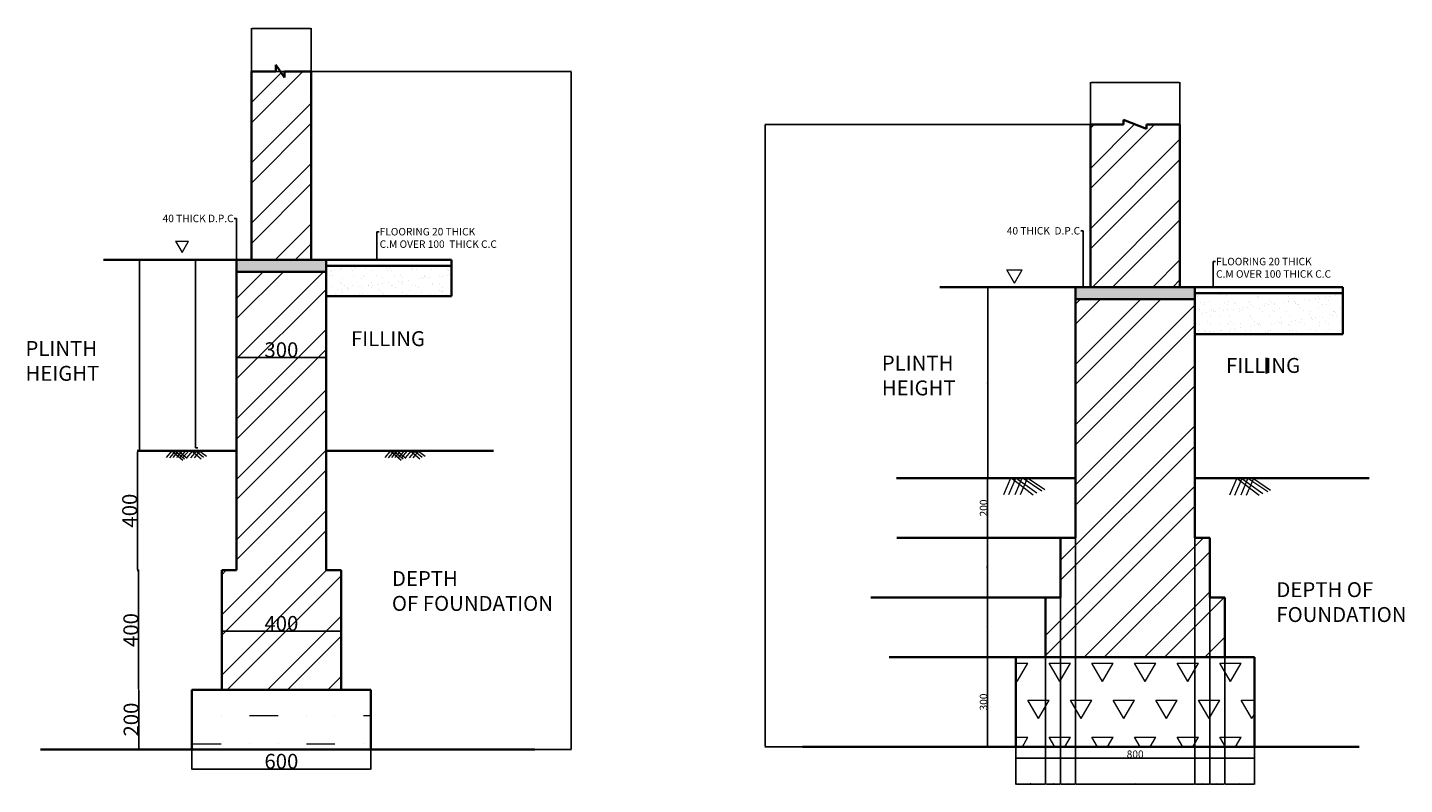
# Model space of a CAD drawing. Units: millimetres. Extents: x 31035 to 42175, y 1348 to 3924.
# Tile 1 of 2: x 31035 to 35648, y 1388 to 3924. Entities that reach past the tile are written whole.
import ezdxf
from ezdxf import colors
from ezdxf.entities.mleader import LeaderData, LeaderLine
from ezdxf.math import Vec2, Vec3

# ---------------------------------------------------------------- set-up
doc = ezdxf.new("R2010")
doc.units = ezdxf.units.MM
for name, color, linetype, lineweight in [('A-ANNO-DIMS', 2, 'Continuous', 18), ('A-ANNO-SYMB', 3, 'Continuous', 18), ('A-ANNO-TEXT', 7, 'Continuous', 18), ('A-SECT', 7, 'Continuous', 35), ('A-WALL-PATT', 8, 'Continuous', 13), ('C-TOPO-PATT', 9, 'Continuous', 13), ('S-FNDN-PATT', 252, 'Continuous', 13)]:
    doc.layers.add(name, color=color, linetype=linetype, lineweight=lineweight)
doc.styles.get("Standard").update_dxf_attribs({"font": 'arial.ttf'})
doc.dimstyles.new('ISO-25', dxfattribs={"dimtxt": 2.5, "dimasz": 2.5, "dimexe": 1.25, "dimexo": 0.625, "dimtad": 1, "dimtxsty": 'Standard', "dimcen": 2.5, "dimadec": 0, "dimazin": 0, "dimtfac": 1, "dimtmove": 0, "dimatfit": 3, "dimfxl": 1, "dimarcsym": 0})
pattern_1 = [(37.5, (28921.223, 0), (-1.60003, 48.94132), [0, -38.608, 0, -43.18, 0, -41.275]), (7.5, (28921.223, 0), (44.9523, 71.6825), [0, -20.828, 0, -34.798, 0, -13.335]), (327.5, (28889.98, 0), (79.09924, 0.14372), [0, -12.7, 0, -45.72, 0, -59.69]), (317.5, (28889.98, 0), (76.35565, 22.29293), [0, -6.35, 0, -29.972, 0, -34.29])]
pattern_2 = [(45, (28921.22, 0), (-101.028, 101.028), []), (45, (28988.58, 0), (-101.028, 101.028), [])]

# ---------------------------------------------------------------- blocks, each defined once
blk = doc.blocks.new('*D1')
at = {"layer": 'A-ANNO-DIMS', "color": 0, "lineweight": -2, "transparency": 16777216}
for p, q in [((31735.2, 2816.7), (31735.2, 2819.2)), ((31737.7, 2818), (32032.7, 2818)), ((32035.2, 2816.7), (32035.2, 2819.2))]:
    blk.add_line(p, q, dxfattribs=at)
at = {"layer": 'A-ANNO-DIMS', "color": 0, "transparency": 16777216}
for points in [[(31737.7, 2818.4), (31737.7, 2817.6), (31735.2, 2818)], [(32032.7, 2818.4), (32032.7, 2817.6), (32035.2, 2818)]]:
    blk.add_solid(points, dxfattribs=at)
at = {"layer": 'Defpoints', "color": 0, "transparency": 16777216}
for p in [(31735.2, 2816.1), (32035.2, 2818), (32035.2, 2816.1)]:
    blk.add_point(p, dxfattribs=at)
at = {"layer": 'A-ANNO-DIMS', "color": 0, "transparency": 16777216, "insert": (31885.2, 2844.1), "char_height": 2.5, "attachment_point": 5}
blk.add_mtext('{\\H20x;300}', dxfattribs=at)
blk = doc.blocks.new('*D2')
at = {"layer": 'A-ANNO-DIMS', "color": 0, "lineweight": -2, "transparency": 16777216}
for p, q in [((31685.2, 1904.6), (31685.2, 1899.9)), ((31687.7, 1901.2), (32082.7, 1901.2)), ((32085.2, 1904.6), (32085.2, 1899.9))]:
    blk.add_line(p, q, dxfattribs=at)
at = {"layer": 'A-ANNO-DIMS', "color": 0, "transparency": 16777216}
for points in [[(31687.7, 1901.6), (31687.7, 1900.8), (31685.2, 1901.2)], [(32082.7, 1901.6), (32082.7, 1900.8), (32085.2, 1901.2)]]:
    blk.add_solid(points, dxfattribs=at)
at = {"layer": 'Defpoints', "color": 0, "transparency": 16777216}
for p in [(31685.2, 1905.2), (32085.2, 1905.2), (32085.2, 1901.2)]:
    blk.add_point(p, dxfattribs=at)
at = {"layer": 'A-ANNO-DIMS', "color": 0, "transparency": 16777216, "insert": (31885.2, 1927.3), "char_height": 2.5, "attachment_point": 5}
blk.add_mtext('{\\H20x;400}', dxfattribs=at)
blk = doc.blocks.new('*D3')
at = {"layer": 'A-ANNO-DIMS', "color": 0, "lineweight": -2, "transparency": 16777216}
for p, q in [((31448.1, 3145.2), (31409.1, 3145.2)), ((31410.3, 3142.7), (31410.3, 2507.7)), ((31448.1, 2505.2), (31409.1, 2505.2))]:
    blk.add_line(p, q, dxfattribs=at)
at = {"layer": 'A-ANNO-DIMS', "color": 0, "transparency": 16777216}
for points in [[(31409.9, 3142.7), (31410.8, 3142.7), (31410.3, 3145.2)], [(31409.9, 2507.7), (31410.8, 2507.7), (31410.3, 2505.2)]]:
    blk.add_solid(points, dxfattribs=at)
at = {"layer": 'Defpoints', "color": 0, "transparency": 16777216}
for p in [(31448.7, 3145.2), (31410.3, 2505.2), (31448.7, 2505.2)]:
    blk.add_point(p, dxfattribs=at)
at = {"layer": 'A-ANNO-DIMS', "color": 0, "transparency": 16777216, "insert": (31408.4, 2825.2), "char_height": 2.5, "attachment_point": 5, "rotation": 90}
blk.add_mtext('640', dxfattribs=at)
blk = doc.blocks.new('*D4')
at = {"layer": 'A-ANNO-DIMS', "color": 0, "lineweight": -2, "transparency": 16777216}
for p, q in [((31408.5, 2505.2), (31401.8, 2505.2)), ((31403.1, 2502.7), (31403.1, 2107.7)), ((31405.4, 2105.2), (31401.8, 2105.2))]:
    blk.add_line(p, q, dxfattribs=at)
at = {"layer": 'A-ANNO-DIMS', "color": 0, "transparency": 16777216}
for points in [[(31402.7, 2502.7), (31403.5, 2502.7), (31403.1, 2505.2)], [(31402.7, 2107.7), (31403.5, 2107.7), (31403.1, 2105.2)]]:
    blk.add_solid(points, dxfattribs=at)
at = {"layer": 'Defpoints', "color": 0, "transparency": 16777216}
for p in [(31409.1, 2505.2), (31403.1, 2105.2), (31406, 2105.2)]:
    blk.add_point(p, dxfattribs=at)
at = {"layer": 'A-ANNO-DIMS', "color": 0, "transparency": 16777216, "insert": (31376.9, 2305.2), "char_height": 2.5, "attachment_point": 5, "rotation": 90}
blk.add_mtext('{\\H20x;400}', dxfattribs=at)
blk = doc.blocks.new('*D5')
at = {"layer": 'A-ANNO-DIMS', "color": 0, "lineweight": -2, "transparency": 16777216}
for p, q in [((31409, 2105.2), (31405.8, 2105.2)), ((31407, 2102.7), (31407, 1707.7)), ((31409, 1705.2), (31405.8, 1705.2))]:
    blk.add_line(p, q, dxfattribs=at)
at = {"layer": 'A-ANNO-DIMS', "color": 0, "transparency": 16777216}
for points in [[(31406.6, 2102.7), (31407.5, 2102.7), (31407, 2105.2)], [(31406.6, 1707.7), (31407.5, 1707.7), (31407, 1705.2)]]:
    blk.add_solid(points, dxfattribs=at)
at = {"layer": 'Defpoints', "color": 0, "transparency": 16777216}
for p in [(31409.6, 2105.2), (31407, 1705.2), (31409.6, 1705.2)]:
    blk.add_point(p, dxfattribs=at)
at = {"layer": 'A-ANNO-DIMS', "color": 0, "transparency": 16777216, "insert": (31380.9, 1905.2), "char_height": 2.5, "attachment_point": 5, "rotation": 90}
blk.add_mtext('{\\H20x;400}', dxfattribs=at)
blk = doc.blocks.new('*D6')
at = {"layer": 'A-ANNO-DIMS', "color": 0, "lineweight": -2, "transparency": 16777216}
for p, q in [((31409, 1705.2), (31406.7, 1705.2)), ((31408, 1702.7), (31408, 1507.7)), ((31409, 1505.2), (31406.7, 1505.2))]:
    blk.add_line(p, q, dxfattribs=at)
at = {"layer": 'A-ANNO-DIMS', "color": 0, "transparency": 16777216}
for points in [[(31407.6, 1702.7), (31408.4, 1702.7), (31408, 1705.2)], [(31407.6, 1507.7), (31408.4, 1507.7), (31408, 1505.2)]]:
    blk.add_solid(points, dxfattribs=at)
at = {"layer": 'Defpoints', "color": 0, "transparency": 16777216}
for p in [(31409.6, 1705.2), (31408, 1505.2), (31409.6, 1505.2)]:
    blk.add_point(p, dxfattribs=at)
at = {"layer": 'A-ANNO-DIMS', "color": 0, "transparency": 16777216, "insert": (31381.8, 1605.2), "char_height": 2.5, "attachment_point": 5, "rotation": 90}
blk.add_mtext('{\\H20x;200}', dxfattribs=at)
blk = doc.blocks.new('*D7')
at = {"layer": 'A-ANNO-DIMS', "color": 0, "lineweight": -2, "transparency": 16777216}
for p, q in [((31585.2, 1504.6), (31585.2, 1438)), ((32185.2, 1504.6), (32185.2, 1438)), ((31587.7, 1439.3), (32182.7, 1439.3))]:
    blk.add_line(p, q, dxfattribs=at)
at = {"layer": 'A-ANNO-DIMS', "color": 0, "transparency": 16777216}
for points in [[(31587.7, 1439.7), (31587.7, 1438.9), (31585.2, 1439.3)], [(32182.7, 1439.7), (32182.7, 1438.9), (32185.2, 1439.3)]]:
    blk.add_solid(points, dxfattribs=at)
at = {"layer": 'Defpoints', "color": 0, "transparency": 16777216}
for p in [(31585.2, 1505.2), (32185.2, 1505.2), (32185.2, 1439.3)]:
    blk.add_point(p, dxfattribs=at)
at = {"layer": 'A-ANNO-DIMS', "color": 0, "transparency": 16777216, "insert": (31885.2, 1465.4), "char_height": 2.5, "attachment_point": 5}
blk.add_mtext('{\\H20x;600}', dxfattribs=at)
blk = doc.blocks.new('*D8')
at = {"layer": 'A-ANNO-DIMS', "color": 0, "lineweight": -2, "transparency": 16777216}
for p, q in [((34340.3, 3054.1), (34250.6, 3054.1)), ((34251.9, 3051.6), (34251.9, 2416.6)), ((34340.3, 2414.1), (34250.6, 2414.1))]:
    blk.add_line(p, q, dxfattribs=at)
at = {"layer": 'A-ANNO-DIMS', "color": 0, "transparency": 16777216}
for points in [[(34251.5, 3051.6), (34252.3, 3051.6), (34251.9, 3054.1)], [(34251.5, 2416.6), (34252.3, 2416.6), (34251.9, 2414.1)]]:
    blk.add_solid(points, dxfattribs=at)
at = {"layer": 'Defpoints', "color": 0, "transparency": 16777216}
for p in [(34341, 3054.1), (34251.9, 2414.1), (34341, 2414.1)]:
    blk.add_point(p, dxfattribs=at)
at = {"layer": 'A-ANNO-DIMS', "color": 0, "transparency": 16777216, "insert": (34250, 2734.1), "char_height": 2.5, "attachment_point": 5, "rotation": 90}
blk.add_mtext('640', dxfattribs=at)
blk = doc.blocks.new('*D9')
at = {"layer": 'A-ANNO-DIMS', "color": 0, "lineweight": -2, "transparency": 16777216}
for p, q in [((34251.2, 2414.1), (34249.6, 2414.1)), ((34250.9, 2411.6), (34250.9, 2216.6)), ((34251.2, 2214.1), (34249.6, 2214.1))]:
    blk.add_line(p, q, dxfattribs=at)
at = {"layer": 'A-ANNO-DIMS', "color": 0, "transparency": 16777216}
for points in [[(34250.4, 2411.6), (34251.3, 2411.6), (34250.9, 2414.1)], [(34250.4, 2216.6), (34251.3, 2216.6), (34250.9, 2214.1)]]:
    blk.add_solid(points, dxfattribs=at)
at = {"layer": 'Defpoints', "color": 0, "transparency": 16777216}
for p in [(34251.9, 2414.1), (34250.9, 2214.1), (34251.9, 2214.1)]:
    blk.add_point(p, dxfattribs=at)
at = {"layer": 'A-ANNO-DIMS', "color": 0, "transparency": 16777216, "insert": (34237.5, 2314.1), "char_height": 2.5, "attachment_point": 5, "rotation": 90}
blk.add_mtext('{\\H10x;200}', dxfattribs=at)
blk = doc.blocks.new('*D10')
at = {"layer": 'A-ANNO-DIMS', "color": 0, "lineweight": -2, "transparency": 16777216}
for p, q in [((34251.1, 2216.6), (34252.1, 2216.6)), ((34250.9, 2214.1), (34250.9, 2016.6)), ((34251.1, 2014.1), (34252.1, 2014.1))]:
    blk.add_line(p, q, dxfattribs=at)
at = {"layer": 'A-ANNO-DIMS', "color": 0, "transparency": 16777216}
for points in [[(34250.4, 2214.1), (34251.3, 2214.1), (34250.9, 2216.6)], [(34250.4, 2016.6), (34251.3, 2016.6), (34250.9, 2014.1)]]:
    blk.add_solid(points, dxfattribs=at)
at = {"layer": 'Defpoints', "color": 0, "transparency": 16777216}
for p in [(34250.4, 2216.6), (34250.4, 2014.1), (34250.9, 2014.1)]:
    blk.add_point(p, dxfattribs=at)
at = {"layer": 'A-ANNO-DIMS', "color": 0, "transparency": 16777216, "insert": (34248.7, 2115.3), "char_height": 2.5, "attachment_point": 5, "rotation": 90}
blk.add_mtext('202,5', dxfattribs=at)
blk = doc.blocks.new('*D11')
at = {"layer": 'A-ANNO-DIMS', "color": 0, "lineweight": -2, "transparency": 16777216}
for p, q in [((34251, 2014.1), (34251, 1816.6)), ((34251.1, 2016.6), (34252.2, 2016.6)), ((34251.1, 1814.1), (34252.2, 1814.1))]:
    blk.add_line(p, q, dxfattribs=at)
at = {"layer": 'A-ANNO-DIMS', "color": 0, "transparency": 16777216}
for points in [[(34250.6, 2014.1), (34251.4, 2014.1), (34251, 2016.6)], [(34250.6, 1816.6), (34251.4, 1816.6), (34251, 1814.1)]]:
    blk.add_solid(points, dxfattribs=at)
at = {"layer": 'Defpoints', "color": 0, "transparency": 16777216}
for p in [(34250.4, 2016.6), (34250.4, 1814.1), (34251, 1814.1)]:
    blk.add_point(p, dxfattribs=at)
at = {"layer": 'A-ANNO-DIMS', "color": 0, "transparency": 16777216, "insert": (34248.9, 1915.3), "char_height": 2.5, "attachment_point": 5, "rotation": 90}
blk.add_mtext('202,5', dxfattribs=at)
blk = doc.blocks.new('*D12')
at = {"layer": 'A-ANNO-DIMS', "color": 0, "lineweight": -2, "transparency": 16777216}
for p, q in [((34250.8, 1811.6), (34250.8, 1516.6)), ((34251.1, 1814.1), (34252.1, 1814.1)), ((34251.1, 1514.1), (34252.1, 1514.1))]:
    blk.add_line(p, q, dxfattribs=at)
at = {"layer": 'A-ANNO-DIMS', "color": 0, "transparency": 16777216}
for points in [[(34250.4, 1811.6), (34251.2, 1811.6), (34250.8, 1814.1)], [(34250.4, 1516.6), (34251.2, 1516.6), (34250.8, 1514.1)]]:
    blk.add_solid(points, dxfattribs=at)
at = {"layer": 'Defpoints', "color": 0, "transparency": 16777216}
for p in [(34250.4, 1814.1), (34250.4, 1514.1), (34250.8, 1514.1)]:
    blk.add_point(p, dxfattribs=at)
at = {"layer": 'A-ANNO-DIMS', "color": 0, "transparency": 16777216, "insert": (34237.4, 1664.1), "char_height": 2.5, "attachment_point": 5, "rotation": 90}
blk.add_mtext('{\\H10x;300}', dxfattribs=at)
blk = doc.blocks.new('*D13')
at = {"layer": 'A-ANNO-DIMS', "color": 0, "lineweight": -2, "transparency": 16777216}
for p, q in [((34345.3, 1513.5), (34345.3, 1474.6)), ((35145.3, 1513.5), (35145.3, 1474.6)), ((34347.8, 1475.8), (35142.8, 1475.8))]:
    blk.add_line(p, q, dxfattribs=at)
at = {"layer": 'A-ANNO-DIMS', "color": 0, "transparency": 16777216}
for points in [[(34347.8, 1476.3), (34347.8, 1475.4), (34345.3, 1475.8)], [(35142.8, 1476.3), (35142.8, 1475.4), (35145.3, 1475.8)]]:
    blk.add_solid(points, dxfattribs=at)
at = {"layer": 'Defpoints', "color": 0, "transparency": 16777216}
for p in [(34345.3, 1514.1), (35145.3, 1514.1), (35145.3, 1475.8)]:
    blk.add_point(p, dxfattribs=at)
at = {"layer": 'A-ANNO-DIMS', "color": 0, "transparency": 16777216, "insert": (34745.3, 1489.2), "char_height": 2.5, "attachment_point": 5}
blk.add_mtext('{\\H10x;800}', dxfattribs=at)
blk = doc.blocks.new('EARTH-SYMBOL-A')
for p, q in [((19.1, 30.7), (0, 8.3)), ((29.8, 30.3), (10.7, 7.9)), ((19.1, 30.7), (55, 0)), ((41.3, 30.7), (22.2, 8.3)), ((29.8, 30.3), (60.9, 4.5)), ((52.9, 30.7), (33.8, 8.3)), ((41.3, 30.7), (69.8, 6.7)), ((63.1, 30.3), (44, 7.9)), ((75.1, 30.7), (56, 8.3)), ((86.6, 29.8), (67.5, 7.5)), ((100.3, 30.3), (81.2, 7.9)), ((86.6, 29.8), (116.9, 4)), ((112.3, 30.3), (93.2, 7.9)), ((100.3, 30.3), (124.7, 10)), ((112.3, 30.3), (134.6, 13.2))]:
    blk.add_line(p, q)
blk = doc.blocks.new('EARTH-SYMBOL-B')
for p, q in [((24.2, 58), (0, 0.7)), ((40.9, 57.3), (16.7, 0)), ((24.2, 58), (99.5, 0.7)), ((61.9, 58), (37.7, 0.7)), ((40.9, 57.3), (111.8, 6.5)), ((80.1, 57.3), (55.9, 0)), ((61.9, 58), (128.5, 13.8)), ((80.1, 57.3), (137.9, 18.1))]:
    blk.add_line(p, q)
blk = doc.blocks.new('*D23')
at = {"layer": 'A-ANNO-DIMS', "color": 0, "lineweight": -2, "transparency": 16777216}
for p, q in [((31785.8, 3776.5), (32856.9, 3776.5)), ((32855.6, 3774), (32855.6, 1507.7)), ((32185.8, 1505.2), (32856.9, 1505.2))]:
    blk.add_line(p, q, dxfattribs=at)
at = {"layer": 'A-ANNO-DIMS', "color": 0, "transparency": 16777216}
for points in [[(32855.2, 3774), (32856.1, 3774), (32855.6, 3776.5)], [(32855.2, 1507.7), (32856.1, 1507.7), (32855.6, 1505.2)]]:
    blk.add_solid(points, dxfattribs=at)
at = {"layer": 'Defpoints', "color": 0, "transparency": 16777216}
for p in [(31785.2, 3776.5), (32185.2, 1505.2), (32855.6, 1505.2)]:
    blk.add_point(p, dxfattribs=at)
at = {"layer": 'A-ANNO-DIMS', "color": 0, "transparency": 16777216, "insert": (32853.7, 2640.9), "char_height": 2.5, "attachment_point": 5, "rotation": 90}
blk.add_mtext('2271.3', dxfattribs=at)
blk = doc.blocks.new('*D24')
at = {"layer": 'A-ANNO-DIMS', "color": 0, "lineweight": -2, "transparency": 16777216}
for p, q in [((34594.6, 3599.3), (33504.9, 3599.3)), ((33506.1, 3596.8), (33506.1, 1516.6)), ((34344.6, 1514.1), (33504.9, 1514.1))]:
    blk.add_line(p, q, dxfattribs=at)
at = {"layer": 'A-ANNO-DIMS', "color": 0, "transparency": 16777216}
for points in [[(33505.7, 3596.8), (33506.5, 3596.8), (33506.1, 3599.3)], [(33505.7, 1516.6), (33506.5, 1516.6), (33506.1, 1514.1)]]:
    blk.add_solid(points, dxfattribs=at)
at = {"layer": 'Defpoints', "color": 0, "transparency": 16777216}
for p in [(34595.3, 3599.3), (33506.1, 1514.1), (34345.3, 1514.1)]:
    blk.add_point(p, dxfattribs=at)
at = {"layer": 'A-ANNO-DIMS', "color": 0, "transparency": 16777216, "insert": (33504.2, 2556.7), "char_height": 2.5, "attachment_point": 5, "rotation": 90}
blk.add_mtext('2085.2', dxfattribs=at)
blk = doc.blocks.new('*D25')
at = {"layer": 'A-ANNO-DIMS', "color": 0, "lineweight": -2, "transparency": 16777216}
for p, q in [((34595.3, 3599.9), (34595.3, 3740.5)), ((34597.8, 3739.3), (34892.8, 3739.3)), ((34895.3, 3599.9), (34895.3, 3740.5))]:
    blk.add_line(p, q, dxfattribs=at)
at = {"layer": 'A-ANNO-DIMS', "color": 0, "transparency": 16777216}
for points in [[(34597.8, 3739.7), (34597.8, 3738.9), (34595.3, 3739.3)], [(34892.8, 3739.7), (34892.8, 3738.9), (34895.3, 3739.3)]]:
    blk.add_solid(points, dxfattribs=at)
at = {"layer": 'Defpoints', "color": 0, "transparency": 16777216}
for p in [(34895.3, 3739.3), (34595.3, 3599.3), (34895.3, 3599.3)]:
    blk.add_point(p, dxfattribs=at)
at = {"layer": 'A-ANNO-DIMS', "color": 0, "transparency": 16777216, "insert": (34745.3, 3741.2), "char_height": 2.5, "attachment_point": 5}
blk.add_mtext('300', dxfattribs=at)
blk = doc.blocks.new('*D38')
at = {"layer": 'A-ANNO-DIMS', "color": 0, "lineweight": -2, "transparency": 16777216}
for p, q in [((34345.3, 1813.5), (34345.3, 1387.8)), ((34445.3, 1813.5), (34445.3, 1387.8)), ((34347.8, 1389.1), (34442.8, 1389.1))]:
    blk.add_line(p, q, dxfattribs=at)
at = {"layer": 'A-ANNO-DIMS', "color": 0, "transparency": 16777216}
for points in [[(34347.8, 1389.5), (34347.8, 1388.7), (34345.3, 1389.1)], [(34442.8, 1389.5), (34442.8, 1388.7), (34445.3, 1389.1)]]:
    blk.add_solid(points, dxfattribs=at)
at = {"layer": 'Defpoints', "color": 0, "transparency": 16777216}
for p in [(34345.3, 1814.1), (34445.3, 1814.1), (34445.3, 1389.1)]:
    blk.add_point(p, dxfattribs=at)
at = {"layer": 'A-ANNO-DIMS', "color": 0, "transparency": 16777216, "insert": (34395.3, 1391), "char_height": 2.5, "attachment_point": 5}
blk.add_mtext('100', dxfattribs=at)
blk = doc.blocks.new('*D39')
at = {"layer": 'A-ANNO-DIMS', "color": 0, "lineweight": -2, "transparency": 16777216}
for p, q in [((34495.3, 2013.5), (34495.3, 1387.8)), ((34445.3, 1813.5), (34445.3, 1387.8)), ((34447.8, 1389.1), (34492.8, 1389.1))]:
    blk.add_line(p, q, dxfattribs=at)
at = {"layer": 'A-ANNO-DIMS', "color": 0, "transparency": 16777216}
for points in [[(34447.8, 1389.5), (34447.8, 1388.7), (34445.3, 1389.1)], [(34492.8, 1389.5), (34492.8, 1388.7), (34495.3, 1389.1)]]:
    blk.add_solid(points, dxfattribs=at)
at = {"layer": 'Defpoints', "color": 0, "transparency": 16777216}
for p in [(34495.3, 2014.1), (34445.3, 1814.1), (34495.3, 1389.1)]:
    blk.add_point(p, dxfattribs=at)
at = {"layer": 'A-ANNO-DIMS', "color": 0, "transparency": 16777216, "insert": (34470.3, 1391), "char_height": 2.5, "attachment_point": 5}
blk.add_mtext('50', dxfattribs=at)
blk = doc.blocks.new('*D40')
at = {"layer": 'A-ANNO-DIMS', "color": 0, "lineweight": -2, "transparency": 16777216}
for p, q in [((34545.3, 2213.5), (34545.3, 1387.8)), ((34495.3, 2013.5), (34495.3, 1387.8)), ((34497.8, 1389.1), (34542.8, 1389.1))]:
    blk.add_line(p, q, dxfattribs=at)
at = {"layer": 'A-ANNO-DIMS', "color": 0, "transparency": 16777216}
for points in [[(34497.8, 1389.5), (34497.8, 1388.7), (34495.3, 1389.1)], [(34542.8, 1389.5), (34542.8, 1388.7), (34545.3, 1389.1)]]:
    blk.add_solid(points, dxfattribs=at)
at = {"layer": 'Defpoints', "color": 0, "transparency": 16777216}
for p in [(34545.3, 2214.1), (34495.3, 2014.1), (34545.3, 1389.1)]:
    blk.add_point(p, dxfattribs=at)
at = {"layer": 'A-ANNO-DIMS', "color": 0, "transparency": 16777216, "insert": (34520.3, 1391), "char_height": 2.5, "attachment_point": 5}
blk.add_mtext('50', dxfattribs=at)
blk = doc.blocks.new('*D41')
at = {"layer": 'A-ANNO-DIMS', "color": 0, "lineweight": -2, "transparency": 16777216}
for p, q in [((34545.3, 2213.5), (34545.3, 1387.8)), ((34945.3, 2213.5), (34945.3, 1387.8)), ((34547.8, 1389.1), (34942.8, 1389.1))]:
    blk.add_line(p, q, dxfattribs=at)
at = {"layer": 'A-ANNO-DIMS', "color": 0, "transparency": 16777216}
for points in [[(34547.8, 1389.5), (34547.8, 1388.7), (34545.3, 1389.1)], [(34942.8, 1389.5), (34942.8, 1388.7), (34945.3, 1389.1)]]:
    blk.add_solid(points, dxfattribs=at)
at = {"layer": 'Defpoints', "color": 0, "transparency": 16777216}
for p in [(34545.3, 2214.1), (34945.3, 2214.1), (34945.3, 1389.1)]:
    blk.add_point(p, dxfattribs=at)
at = {"layer": 'A-ANNO-DIMS', "color": 0, "transparency": 16777216, "insert": (34745.3, 1391), "char_height": 2.5, "attachment_point": 5}
blk.add_mtext('400', dxfattribs=at)
blk = doc.blocks.new('*D42')
at = {"layer": 'A-ANNO-DIMS', "color": 0, "lineweight": -2, "transparency": 16777216}
for p, q in [((34945.3, 2213.5), (34945.3, 1387.8)), ((34995.3, 2013.5), (34995.3, 1387.8)), ((34947.8, 1389.1), (34992.8, 1389.1))]:
    blk.add_line(p, q, dxfattribs=at)
at = {"layer": 'A-ANNO-DIMS', "color": 0, "transparency": 16777216}
for points in [[(34947.8, 1389.5), (34947.8, 1388.7), (34945.3, 1389.1)], [(34992.8, 1389.5), (34992.8, 1388.7), (34995.3, 1389.1)]]:
    blk.add_solid(points, dxfattribs=at)
at = {"layer": 'Defpoints', "color": 0, "transparency": 16777216}
for p in [(34945.3, 2214.1), (34995.3, 2014.1), (34995.3, 1389.1)]:
    blk.add_point(p, dxfattribs=at)
at = {"layer": 'A-ANNO-DIMS', "color": 0, "transparency": 16777216, "insert": (34970.3, 1391), "char_height": 2.5, "attachment_point": 5}
blk.add_mtext('50', dxfattribs=at)
blk = doc.blocks.new('*D43')
at = {"layer": 'A-ANNO-DIMS', "color": 0, "lineweight": -2, "transparency": 16777216}
for p, q in [((34995.3, 2013.5), (34995.3, 1387.8)), ((35045.3, 1813.5), (35045.3, 1387.8)), ((34997.8, 1389.1), (35042.8, 1389.1))]:
    blk.add_line(p, q, dxfattribs=at)
at = {"layer": 'A-ANNO-DIMS', "color": 0, "transparency": 16777216}
for points in [[(34997.8, 1389.5), (34997.8, 1388.7), (34995.3, 1389.1)], [(35042.8, 1389.5), (35042.8, 1388.7), (35045.3, 1389.1)]]:
    blk.add_solid(points, dxfattribs=at)
at = {"layer": 'Defpoints', "color": 0, "transparency": 16777216}
for p in [(34995.3, 2014.1), (35045.3, 1814.1), (35045.3, 1389.1)]:
    blk.add_point(p, dxfattribs=at)
at = {"layer": 'A-ANNO-DIMS', "color": 0, "transparency": 16777216, "insert": (35020.3, 1391), "char_height": 2.5, "attachment_point": 5}
blk.add_mtext('50', dxfattribs=at)
blk = doc.blocks.new('*D44')
at = {"layer": 'A-ANNO-DIMS', "color": 0, "lineweight": -2, "transparency": 16777216}
for p, q in [((35045.3, 1813.5), (35045.3, 1387.8)), ((35145.3, 1813.5), (35145.3, 1387.8)), ((35047.8, 1389.1), (35142.8, 1389.1))]:
    blk.add_line(p, q, dxfattribs=at)
at = {"layer": 'A-ANNO-DIMS', "color": 0, "transparency": 16777216}
for points in [[(35047.8, 1389.5), (35047.8, 1388.7), (35045.3, 1389.1)], [(35142.8, 1389.5), (35142.8, 1388.7), (35145.3, 1389.1)]]:
    blk.add_solid(points, dxfattribs=at)
at = {"layer": 'Defpoints', "color": 0, "transparency": 16777216}
for p in [(35045.3, 1814.1), (35145.3, 1814.1), (35145.3, 1389.1)]:
    blk.add_point(p, dxfattribs=at)
at = {"layer": 'A-ANNO-DIMS', "color": 0, "transparency": 16777216, "insert": (35095.3, 1391), "char_height": 2.5, "attachment_point": 5}
blk.add_mtext('100', dxfattribs=at)
blk = doc.blocks.new('*D54')
at = {"layer": 'A-ANNO-DIMS', "color": 0, "lineweight": -2, "transparency": 16777216}
for p, q in [((31785.2, 3777.1), (31785.2, 3921.4)), ((31985.2, 3777.1), (31985.2, 3921.4)), ((31787.7, 3920.2), (31982.7, 3920.2))]:
    blk.add_line(p, q, dxfattribs=at)
at = {"layer": 'A-ANNO-DIMS', "color": 0, "transparency": 16777216}
for points in [[(31787.7, 3920.6), (31787.7, 3919.7), (31785.2, 3920.2)], [(31982.7, 3920.6), (31982.7, 3919.7), (31985.2, 3920.2)]]:
    blk.add_solid(points, dxfattribs=at)
at = {"layer": 'Defpoints', "color": 0, "transparency": 16777216}
for p in [(31985.2, 3920.2), (31785.2, 3776.5), (31985.2, 3776.5)]:
    blk.add_point(p, dxfattribs=at)
at = {"layer": 'A-ANNO-DIMS', "color": 0, "transparency": 16777216, "insert": (31885.2, 3922.1), "char_height": 2.5, "attachment_point": 5}
blk.add_mtext('200.0', dxfattribs=at)

msp = doc.modelspace()

# ---------------------------------------------------------------- hatches: boundary and pattern name
at = {"layer": 'A-WALL-PATT'}
h = msp.add_hatch(dxfattribs=at)
h.set_pattern_fill('ANSI32', color=256, scale=15)
h.set_pattern_definition(pattern_2)
h.paths.add_polyline_path([(31985.18, 3776.491), (31895.377, 3776.491), (31895.377, 3755.844), (31866.299, 3799.154), (31866.299, 3776.491), (31785.18, 3776.491), (31785.18, 3145.234), (31985.18, 3145.234)])
h = msp.add_hatch(dxfattribs=at)
h.set_pattern_fill('ANSI32', color=256, scale=15)
h.set_pattern_definition(pattern_2)
h.paths.add_polyline_path([(34595.269, 3054.088), (34895.269, 3054.088), (34895.269, 3599.312), (34783.558, 3599.312), (34783.558, 3584.35), (34706.677, 3614.273), (34706.677, 3599.312), (34595.269, 3599.312)])
h = msp.add_hatch(color=256, dxfattribs=at)
h.dxf.hatch_style = 1
h.paths.add_polyline_path([(32035.18, 3145.234), (31735.18, 3145.234), (31735.18, 3105.234), (32035.18, 3105.234)])
h = msp.add_hatch(dxfattribs=at)
h.set_pattern_fill('ANSI32', color=256, scale=15)
h.set_pattern_definition(pattern_2)
h.paths.add_polyline_path([(32035.18, 3105.234), (31735.18, 3105.234), (31735.18, 2105.234), (31685.18, 2105.234), (31685.18, 1705.234), (32085.18, 1705.234), (32085.18, 2105.234), (32035.18, 2105.234)])
h.paths.add_polyline_path([(31826.489, 2804.053), (31944.28, 2804.053), (31944.28, 2883.339), (31826.489, 2883.339)], flags=24)
h.paths.add_polyline_path([(31827.512, 1887.238), (31945.304, 1887.238), (31945.304, 1966.524), (31827.512, 1966.524)], flags=24)
h = msp.add_hatch(color=256, dxfattribs=at)
h.dxf.hatch_style = 1
h.paths.add_polyline_path([(34945.269, 3054.088), (34545.269, 3054.088), (34545.269, 3014.088), (34945.269, 3014.088)])
h = msp.add_hatch(dxfattribs=at)
h.set_pattern_fill('ANSI32', color=256, scale=15)
h.set_pattern_definition(pattern_2)
h.paths.add_polyline_path([(34945.269, 3014.088), (34545.269, 3014.088), (34545.269, 2414.088), (34545.269, 2214.088), (34495.269, 2214.088), (34495.269, 2014.088), (34445.269, 2014.088), (34445.269, 1814.088), (35045.269, 1814.088), (35045.269, 2014.088), (34995.269, 2014.088), (34995.269, 2214.088), (34945.269, 2214.088), (34945.269, 2414.088)])
at = {"layer": 'C-TOPO-PATT'}
h = msp.add_hatch(dxfattribs=at)
h.set_pattern_fill('AR-SAND', color=256)
h.set_pattern_definition(pattern_1)
h.paths.add_polyline_path([(32455.406, 3023.971), (32455.406, 3125.234), (32305.678, 3125.234), (32035.18, 3125.234), (32035.18, 3023.971)])
h = msp.add_hatch(dxfattribs=at)
h.set_pattern_fill('AR-SAND', color=256)
h.set_pattern_definition(pattern_1)
h.paths.add_polyline_path([(34945.269, 3034.088), (34945.269, 3014.088), (34945.269, 2896.734), (35441.377, 2896.734), (35441.377, 3034.088)])
at = {"layer": 'S-FNDN-PATT'}
h = msp.add_hatch(dxfattribs=at)
h.set_pattern_fill('TRIANG', color=256, scale=15)
h.set_pattern_definition([(60, (28921.22, 0), (-71.4375, 123.7334), [71.4375, -71.4375]), (120, (28921.22, 0), (-142.875, 8e-08), [71.4375, -71.4375]), (0, (28885.5, 61.87), (71.4375, 123.7334), [71.4375, -71.4375])])
h.paths.add_polyline_path([(34445.269, 1814.088), (34345.269, 1814.088), (34345.269, 1514.088), (35145.269, 1514.088), (35145.269, 1814.088), (35045.269, 1814.088)])
h = msp.add_hatch(dxfattribs=at)
h.set_pattern_fill('MUDST', color=256, scale=15)
h.set_pattern_definition([(0, (28921.22, 0), (190.5, 95.25), [95.25, -95.25, 0, -95.25, 0, -95.25])])
h.paths.add_polyline_path([(32185.18, 1505.234), (32185.18, 1705.234), (31585.18, 1705.234), (31585.18, 1505.234)])

# ---------------------------------------------------------------- linework, layer by layer
at = {"layer": 'A-ANNO-SYMB'}
for p, q in [((31530.86, 3208.547), (31552.684, 3170.398)), ((31552.684, 3170.398), (31574.509, 3208.547)), ((34341.319, 3067.353), (34315.474, 3111.861)), ((34341.319, 3067.353), (34367.164, 3111.861))]:
    msp.add_line(p, q, dxfattribs=at)
for points in [[(31530.86, 3208.547), (31574.509, 3208.547)], [(34315.474, 3111.861), (34367.164, 3111.861)]]:
    msp.add_lwpolyline(points, dxfattribs=at)
at = {"layer": 'A-SECT'}
for p, q in [((31866.299, 3799.154), (31866.299, 3776.491)), ((31866.299, 3799.154), (31895.377, 3755.844)), ((31785.18, 3145.234), (31785.18, 3776.491)), ((31785.18, 3776.491), (31866.299, 3776.491)), ((31895.377, 3776.491), (31895.377, 3755.844)), ((31895.377, 3776.491), (31985.18, 3776.491)), ((31985.18, 3145.234), (31985.18, 3776.491)), ((34595.269, 3054.088), (34595.269, 3599.312)), ((34595.269, 3599.312), (34706.677, 3599.312)), ((34706.677, 3614.273), (34706.677, 3599.312)), ((34706.677, 3614.273), (34783.558, 3584.35)), ((34783.558, 3599.312), (34783.558, 3584.35)), ((34783.558, 3599.312), (34895.269, 3599.312)), ((34895.269, 3054.088), (34895.269, 3599.312)), ((31735.18, 3145.234), (31289.22, 3145.234)), ((31735.18, 2105.234), (31735.18, 3145.234)), ((31735.18, 3145.234), (32035.18, 3145.234)), ((32035.18, 2105.234), (32035.18, 3145.234)), ((32035.18, 3145.234), (32455.406, 3145.234)), ((32455.406, 3145.234), (32455.406, 3023.971)), ((31735.18, 3105.234), (32035.18, 3105.234)), ((32035.18, 3125.234), (32305.678, 3125.234)), ((32305.678, 3125.234), (32455.406, 3125.234)), ((34545.269, 3054.088), (34091.304, 3054.088)), ((34545.269, 3054.088), (34945.269, 3054.088)), ((34545.269, 3014.088), (34545.269, 3054.088)), ((34945.269, 3054.088), (34945.269, 3014.088)), ((34945.269, 3054.088), (35441.377, 3054.088)), ((35441.377, 2896.734), (35441.377, 3054.088)), ((32035.18, 3023.971), (32455.406, 3023.971)), ((34545.269, 2414.088), (34545.269, 3014.088)), ((34545.269, 3014.088), (34945.269, 3014.088)), ((34945.269, 3034.088), (35441.377, 3034.088)), ((34945.269, 3014.088), (34945.269, 2414.088)), ((34945.269, 2896.734), (35441.377, 2896.734)), ((35185.24, 2816.599), (35185.24, 2764.894)), ((31735.18, 2505.234), (31401.822, 2505.234)), ((32035.18, 2505.234), (32085.18, 2505.234)), ((32085.18, 2505.234), (32596.139, 2505.234)), ((34545.269, 2414.088), (33945.447, 2414.088)), ((34545.269, 2414.088), (34545.269, 2214.088)), ((34945.269, 2414.088), (34945.269, 2214.088)), ((34945.269, 2414.088), (35529.266, 2414.088)), ((34495.269, 2214.088), (33946.558, 2214.088)), ((34545.269, 2214.088), (34495.269, 2214.088)), ((34495.269, 2214.088), (34495.269, 2014.088)), ((34945.269, 2214.088), (34995.269, 2214.088)), ((34995.269, 2214.088), (34995.269, 2014.088)), ((31406.154, 2105.234), (31405.791, 2105.234)), ((31685.18, 1705.234), (31685.18, 2105.234)), ((31685.18, 2105.234), (31735.18, 2105.234)), ((32035.18, 2105.234), (32085.18, 2105.234)), ((32085.18, 1705.234), (32085.18, 2105.234)), ((34445.269, 2014.088), (33860.219, 2014.088)), ((34445.269, 1814.088), (34445.269, 2014.088)), ((34445.269, 2014.088), (34495.269, 2014.088)), ((34995.269, 2014.088), (35045.269, 2014.088)), ((35045.269, 1814.088), (35045.269, 2014.088)), ((34345.269, 1814.088), (33920.851, 1814.088)), ((34345.269, 1814.088), (34345.269, 1514.088)), ((34445.269, 1814.088), (34345.269, 1814.088)), ((34445.269, 1814.088), (35045.269, 1814.088)), ((35145.269, 1814.088), (35045.269, 1814.088)), ((35145.269, 1514.088), (35145.269, 1814.088)), ((31585.18, 1505.234), (31585.18, 1705.234)), ((31585.18, 1705.234), (32185.18, 1705.234)), ((32185.18, 1705.234), (32185.18, 1505.234)), ((31585.18, 1505.234), (31078.48, 1505.234)), ((31585.18, 1505.234), (32185.18, 1505.234)), ((32185.18, 1505.234), (32734.646, 1505.234)), ((34345.269, 1514.088), (33631.121, 1514.088)), ((34345.269, 1514.088), (35145.269, 1514.088)), ((35145.269, 1514.088), (35496.017, 1514.088))]:
    msp.add_line(p, q, dxfattribs=at)

# ---------------------------------------------------------------- block references
at = {"layer": 'A-ANNO-SYMB'}
for name, p in [('EARTH-SYMBOL-A', (31499.564, 2474.541)), ('EARTH-SYMBOL-A', (32231.93, 2474.541)), ('EARTH-SYMBOL-B', (34304.501, 2357.941)), ('EARTH-SYMBOL-B', (35061.282, 2356.047))]:
    msp.add_blockref(name, p, dxfattribs=at)

# ---------------------------------------------------------------- texts
at = {"layer": 'A-ANNO-TEXT', "char_height": 50, "attachment_point": 1}
for s, width, insert in [('FILLING', 135.33088, (32118.193, 2906.361)), ('PLINTH  HEIGHT ', 135.33088, (31027.899, 2873.567)), ('PLINTH  HEIGHT ', 135.33088, (33896.526, 2824.685)), ('FILLING', 135.33088, (35049.909, 2816.599)), ('DEPTH \\POF FOUNDATION', 677.66591, (32255.441, 2102.805)), ('DEPTH OF FOUNDATION', 737.29352, (35218.471, 2065.45))]:
    msp.add_mtext_dynamic_manual_height_columns(s, width=width, gutter_width=12.5, heights=[0], dxfattribs=dict(at, insert=insert))

# ---------------------------------------------------------------- dimensions: what is measured, and where the dimension line sits
at = {"layer": 'A-ANNO-DIMS'}
for base, p1, p2, override, picture, middle in [((31985.18, 3920.154), (31785.18, 3776.491), (31985.18, 3776.491), {"dimdec": 1, "dimlfac": 1, "dimrnd": 0, "dimzin": 0, "dimdsep": 46, "dimlunit": 2}, '*D54', (31885.18, 3922.056)), ((34895.269, 3739.273), (34595.269, 3599.312), (34895.269, 3599.312), {"dimdec": 0, "dimlfac": 1, "dimrnd": 0, "dimzin": 0, "dimdsep": 46, "dimlunit": 2}, '*D25', (34745.269, 3741.175)), ((34545.269, 1389.088), (34495.269, 2014.088), (34545.269, 2214.088), {"dimdec": 0, "dimlfac": 1, "dimrnd": 0, "dimzin": 0, "dimdsep": 46, "dimlunit": 2}, '*D40', (34520.269, 1390.989)), ((34945.269, 1389.088), (34545.269, 2214.088), (34945.269, 2214.088), {"dimdec": 0, "dimlfac": 1, "dimrnd": 0, "dimzin": 0, "dimdsep": 46, "dimlunit": 2}, '*D41', (34745.269, 1390.989)), ((34995.269, 1389.088), (34945.269, 2214.088), (34995.269, 2014.088), {"dimdec": 0, "dimlfac": 1, "dimrnd": 0, "dimzin": 0, "dimdsep": 46, "dimlunit": 2}, '*D42', (34970.269, 1390.989)), ((34495.269, 1389.088), (34445.269, 1814.088), (34495.269, 2014.088), {"dimdec": 0, "dimlfac": 1, "dimrnd": 0, "dimzin": 0, "dimdsep": 46, "dimlunit": 2}, '*D39', (34470.269, 1390.989)), ((35045.269, 1389.088), (34995.269, 2014.088), (35045.269, 1814.088), {"dimdec": 0, "dimlfac": 1, "dimrnd": 0, "dimzin": 0, "dimdsep": 46, "dimlunit": 2}, '*D43', (35020.269, 1390.989)), ((34445.269, 1389.088), (34345.269, 1814.088), (34445.269, 1814.088), {"dimdec": 0, "dimlfac": 1, "dimrnd": 0, "dimzin": 0, "dimdsep": 46, "dimlunit": 2}, '*D38', (34395.269, 1390.989)), ((35145.269, 1389.088), (35045.269, 1814.088), (35145.269, 1814.088), {"dimdec": 0, "dimlfac": 1, "dimrnd": 0, "dimzin": 0, "dimdsep": 46, "dimlunit": 2}, '*D44', (35095.269, 1390.989))]:
    dim = msp.add_linear_dim(base=base, p1=p1, p2=p2, dimstyle='ISO-25', override=override, dxfattribs=at)
    dim.commit()
    dim.dimension.update_dxf_attribs({"geometry": picture, "text_midpoint": middle})
for base, p1, p2, override, picture, middle in [((32855.646, 1505.234), (31785.18, 3776.491), (32185.18, 1505.234), {"dimdec": 1, "dimlfac": 1, "dimrnd": 0, "dimzin": 0, "dimdsep": 46, "dimlunit": 2}, '*D23', (32853.743, 2640.863)), ((33506.121, 1514.088), (34595.269, 3599.312), (34345.269, 1514.088), {"dimdec": 1, "dimlfac": 1, "dimrnd": 0, "dimzin": 0, "dimdsep": 46, "dimlunit": 2}, '*D24', (33504.22, 2556.7)), ((31410.342, 2505.234), (31448.739, 3145.234), (31448.739, 2505.234), {"dimclrd": 0, "dimclre": 0, "dimclrt": 0}, '*D3', (31408.441, 2825.234)), ((34251.869, 2414.088), (34340.961, 3054.088), (34340.961, 2414.088), {"dimclrd": 0, "dimclre": 0, "dimclrt": 0}, '*D8', (34249.968, 2734.088)), ((34250.865, 2014.088), (34250.44, 2216.588), (34250.44, 2014.088), {"dimclrd": 0, "dimclre": 0, "dimclrt": 0}, '*D10', (34248.738, 2115.338)), ((34250.998, 1814.088), (34250.449, 2016.588), (34250.449, 1814.088), {"dimclrd": 0, "dimclre": 0, "dimclrt": 0}, '*D11', (34248.871, 1915.338))]:
    dim = msp.add_linear_dim(base=base, p1=p1, p2=p2, angle=90, dimstyle='ISO-25', override=override, dxfattribs=at)
    dim.commit()
    dim.dimension.update_dxf_attribs({"geometry": picture, "text_midpoint": middle})
for base, p1, p2, text, picture, middle in [((32035.18, 2817.969), (31735.18, 2816.055), (32035.18, 2816.055), '{\\H20x;<>}', '*D1', (31885.18, 2844.139)), ((32085.18, 1901.188), (31685.18, 1905.234), (32085.18, 1905.234), '{\\H20x;<>}', '*D2', (31885.18, 1927.341)), ((35145.269, 1475.835), (34345.269, 1514.088), (35145.269, 1514.088), '{\\H10x;<>}', '*D13', (34745.269, 1489.224))]:
    dim = msp.add_linear_dim(base=base, p1=p1, p2=p2, text=text, dimstyle='ISO-25', override={"dimclrd": 0, "dimclre": 0, "dimclrt": 0}, dxfattribs=at)
    dim.commit()
    dim.dimension.update_dxf_attribs({"geometry": picture, "text_midpoint": middle})
dim = msp.add_linear_dim(base=(31403.072, 2105.234), p1=(31409.092, 2505.234), p2=(31406.01, 2105.234), angle=90, text='{\\H20x;<>}', dimstyle='ISO-25', override={"dimclrd": 0, "dimclre": 0, "dimclrt": 0}, dxfattribs=at)
dim.commit()
dim.dimension.update_dxf_attribs({"geometry": '*D4', "text_midpoint": (31403.072, 2305.234), "dimtype": 160})
for base, p1, p2, text, picture, middle in [((34250.856, 2214.088), (34251.869, 2414.088), (34251.869, 2214.088), '{\\H10x;<>}', '*D9', (34237.467, 2314.088)), ((31407.041, 1705.234), (31409.579, 2105.234), (31409.579, 1705.234), '{\\H20x;<>}', '*D5', (31380.887, 1905.234)), ((34250.803, 1514.088), (34250.449, 1814.088), (34250.449, 1514.088), '{\\H10x;<>}', '*D12', (34237.405, 1664.088)), ((31407.976, 1505.234), (31409.579, 1705.234), (31409.579, 1505.234), '{\\H20x;<>}', '*D6', (31381.822, 1605.234))]:
    dim = msp.add_linear_dim(base=base, p1=p1, p2=p2, angle=90, text=text, dimstyle='ISO-25', override={"dimclrd": 0, "dimclre": 0, "dimclrt": 0}, dxfattribs=at)
    dim.commit()
    dim.dimension.update_dxf_attribs({"geometry": picture, "text_midpoint": middle})
dim = msp.add_linear_dim(base=(32185.18, 1439.291), p1=(31585.18, 1505.234), p2=(32185.18, 1505.234), text='{\\H20x;<>}', dimstyle='ISO-25', override={"dimclrd": 0, "dimclre": 0, "dimclrt": 0}, dxfattribs=at)
dim.commit()
dim.dimension.update_dxf_attribs({"geometry": '*D7', "text_midpoint": (31885.18, 1439.291), "dimtype": 160})

# ---------------------------------------------------------------- leaders
at = {"layer": 'A-ANNO-TEXT'}
ml = msp.add_multileader_mtext('Standard', dxfattribs=at)
ml.set_content('40 THICK D.P.C', color=256)
ml.set_leader_properties()
ml.build(insert=Vec2(0, 0))
ctx = ml.context
ctx.base_point, ctx.char_height, ctx.plane_origin = Vec3(31468.831, 3283.861), 25, Vec3(31735.18, 3145.234)
ctx.text_align_type = 2
notes = []
notes.append((ctx, [(0, (1, 1, 0), (31735.18, 3283.861), (-1, 0), 8, [(0, [(31735.18, 3145.234)], 0, [])])]))
ctx.mtext.insert, ctx.mtext.alignment, ctx.mtext.flow_direction = Vec3(31725.18, 3296.574), 3, 5
ml = msp.add_multileader_mtext('Standard', dxfattribs=at)
ml.set_content('FLOORING 20 THICK \\PC.M OVER 100  THICK C.C', color=256)
ml.set_leader_properties()
ml.build(insert=Vec2(0, 0))
ctx = ml.context
ctx.base_point, ctx.char_height, ctx.plane_origin = Vec3(32212.489, 3239.547), 25, Vec3(32204.489, 3145.234)
notes.append((ctx, [(0, (1, 1, 0), (32204.489, 3239.547), (1, 0), 8, [(0, [(32204.489, 3145.234)], 0, [])])]))
ctx.mtext.insert, ctx.mtext.flow_direction = Vec3(32214.489, 3252.26), 5
ml = msp.add_multileader_mtext('Standard', dxfattribs=at)
ml.set_content('40 THICK  D.P.C', color=256)
ml.set_leader_properties()
ml.build(insert=Vec2(0, 0))
ctx = ml.context
ctx.base_point, ctx.char_height, ctx.plane_origin = Vec3(34294.821, 3242.6), 25, Vec3(34570.873, 3054.088)
ctx.text_align_type = 2
notes.append((ctx, [(0, (1, 1, 0), (34570.873, 3242.6), (-1, 0), 8, [(0, [(34570.873, 3054.088)], 0, [])])]))
ctx.mtext.insert, ctx.mtext.alignment, ctx.mtext.flow_direction = Vec3(34560.873, 3255.313), 3, 5
ml = msp.add_multileader_mtext('Standard', dxfattribs=at)
ml.set_content('', color=256)
ml.set_leader_properties()
ml.build(insert=Vec2(0, 0))
ctx = ml.context
ctx.base_point, ctx.plane_origin = Vec3(31605.66, 2515.619), Vec3(31597.66, 3145.234)
notes.append((ctx, [(0, (1, 1, 0), (31597.66, 2515.619), (1, 0), 8, [(0, [(31597.66, 3145.234)], 0, [])])]))
ctx.mtext.insert, ctx.mtext.flow_direction = Vec3(31607.66, 2517.619), 5
ml = msp.add_multileader_mtext('Standard', dxfattribs=at)
ml.set_content('FLOORING 20 THICK \\PC.M OVER 100 THICK C.C', color=256)
ml.set_leader_properties()
ml.build(insert=Vec2(0, 0))
ctx = ml.context
ctx.base_point, ctx.char_height, ctx.plane_origin = Vec3(35014.537, 3139.521), 25, Vec3(35006.537, 3054.088)
notes.append((ctx, [(0, (1, 1, 0), (35006.537, 3139.521), (1, 0), 8, [(0, [(35006.537, 3054.088)], 0, [])])]))
ctx.mtext.insert, ctx.mtext.flow_direction = Vec3(35016.537, 3152.234), 5
for ctx, leaders in notes:
    for number, flags, end, landing, length, lines in leaders:
        leader = LeaderData()
        leader.index, (leader.has_last_leader_line, leader.has_dogleg_vector, leader.attachment_direction) = number, flags
        leader.last_leader_point, leader.dogleg_vector, leader.dogleg_length = Vec3(end), Vec3(landing), length
        for number, points, colour, breaks in lines:
            line = LeaderLine()
            line.index, line.vertices, line.color, line.breaks = number, Vec3.list(points), colors.encode_raw_color(colour), breaks
            leader.lines.append(line)
        ctx.leaders.append(leader)

doc.saveas('drawing.dxf')
